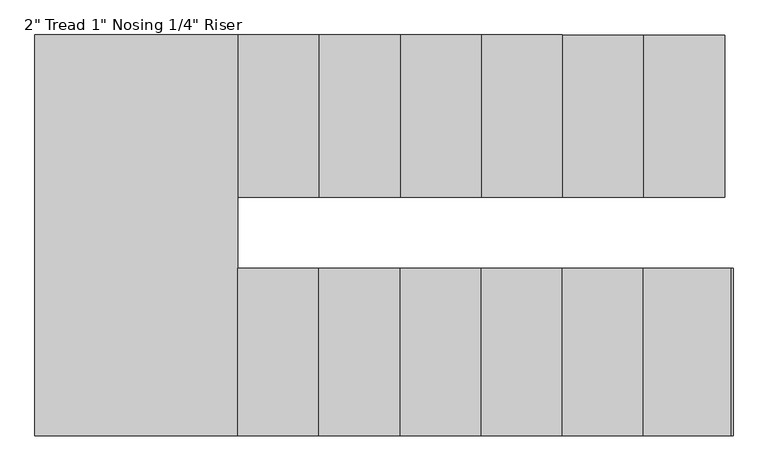
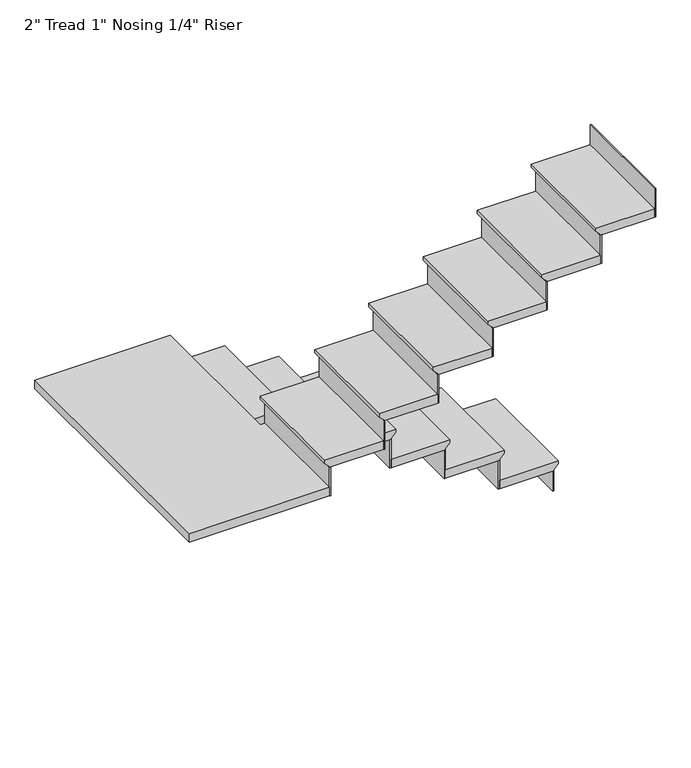
"""IFC4 building model written with IfcOpenShell, lengths in millimetres: stair flight geometry."""

from ifc_helpers import new_model, si_unit, origin, place, context, project, spatial, faceted_brep, source, transform, mapped, element, save


def stair_flight_6f8696f7(model_context):
    return source(origin(), model_context, "Body", "Brep", [
        faceted_brep([(-2968.8120155, -2170.0065691, 6551.0833333), (-2968.8120155, -2170.0065691, 6570.1333333), (-2968.8120155, -2779.6065691, 6570.1333333), (-2968.8120155, -2779.6065691, 6551.0833333), (-2994.2120155, -2170.0065691, 6525.6833333), (-2994.2120155, -2779.6065691, 6525.6833333), (-3299.0120155, -2170.0065691, 6570.1333333), (-3299.0120155, -2779.6065691, 6570.1333333), (-2994.2120155, -2779.6065691, 6519.3333333), (-3299.0120155, -2779.6065691, 6519.3333333), (-3299.0120155, -2170.0065691, 6519.3333333), (-2994.2120155, -2170.0065691, 6519.3333333)], [[[0, 1, 2, 3]], [[4, 0, 3, 5]], [[2, 1, 6, 7]], [[8, 9, 10, 11]], [[2, 7, 9, 8, 5, 3]], [[8, 11, 4, 5]], [[6, 1, 0, 4, 11, 10]], [[7, 6, 10, 9]]]),
        faceted_brep([(-2994.2120155, -2170.0065691, 6519.3333333), (-2994.2120155, -2170.0065691, 6400.8), (-3000.5620155, -2170.0065691, 6400.8), (-3000.5620155, -2170.0065691, 6519.3333333), (-2994.2120155, -2779.6065691, 6519.3333333), (-3000.5620155, -2779.6065691, 6519.3333333), (-3000.5620155, -2779.6065691, 6400.8), (-2994.2120155, -2779.6065691, 6400.8)], [[[0, 1, 2, 3]], [[4, 5, 6, 7]], [[1, 0, 4, 7]], [[2, 1, 7, 6]], [[3, 2, 6, 5]], [[0, 3, 5, 4]]]),
        faceted_brep([(-3299.0120155, -2170.0065691, 6688.6666667), (-3299.0120155, -2170.0065691, 6519.3333333), (-3305.3620155, -2170.0065691, 6519.3333333), (-3305.3620155, -2170.0065691, 6688.6666667), (-3299.0120155, -2779.6065691, 6688.6666667), (-3305.3620155, -2779.6065691, 6688.6666667), (-3305.3620155, -2779.6065691, 6519.3333333), (-3299.0120155, -2779.6065691, 6519.3333333)], [[[0, 1, 2, 3]], [[4, 5, 6, 7]], [[1, 0, 4, 7]], [[2, 1, 7, 6]], [[3, 2, 6, 5]], [[0, 3, 5, 4]]]),
        faceted_brep([(-3273.6120155, -2779.6065691, 6739.4666667), (-3273.6120155, -2170.0065691, 6739.4666667), (-3603.8120155, -2170.0065691, 6739.4666667), (-3603.8120155, -2779.6065691, 6739.4666667), (-3299.0120155, -2779.6065691, 6688.6666667), (-3603.8120155, -2779.6065691, 6688.6666667), (-3603.8120155, -2170.0065691, 6688.6666667), (-3299.0120155, -2170.0065691, 6688.6666667), (-3299.0120155, -2779.6065691, 6695.0166667), (-3273.6120155, -2779.6065691, 6720.4166667), (-3299.0120155, -2170.0065691, 6695.0166667), (-3273.6120155, -2170.0065691, 6720.4166667)], [[[0, 1, 2, 3]], [[4, 5, 6, 7]], [[0, 3, 5, 4, 8, 9]], [[4, 7, 10, 8]], [[2, 1, 11, 10, 7, 6]], [[3, 2, 6, 5]], [[11, 1, 0, 9]], [[10, 11, 9, 8]]]),
        faceted_brep([(-3603.8120155, -2170.0065691, 6858.0), (-3603.8120155, -2170.0065691, 6688.6666667), (-3610.1620155, -2170.0065691, 6688.6666667), (-3610.1620155, -2170.0065691, 6858.0), (-3603.8120155, -2779.6065691, 6858.0), (-3610.1620155, -2779.6065691, 6858.0), (-3610.1620155, -2779.6065691, 6688.6666667), (-3603.8120155, -2779.6065691, 6688.6666667)], [[[0, 1, 2, 3]], [[4, 5, 6, 7]], [[1, 0, 4, 7]], [[2, 1, 7, 6]], [[3, 2, 6, 5]], [[0, 3, 5, 4]]]),
        faceted_brep([(-3578.4120155, -2779.6065691, 6908.8), (-3578.4120155, -2170.0065691, 6908.8), (-3908.6120155, -2170.0065691, 6908.8), (-3908.6120155, -2779.6065691, 6908.8), (-3603.8120155, -2779.6065691, 6858.0), (-3908.6120155, -2779.6065691, 6858.0), (-3908.6120155, -2170.0065691, 6858.0), (-3603.8120155, -2170.0065691, 6858.0), (-3603.8120155, -2779.6065691, 6864.35), (-3578.4120155, -2779.6065691, 6889.75), (-3603.8120155, -2170.0065691, 6864.35), (-3578.4120155, -2170.0065691, 6889.75)], [[[0, 1, 2, 3]], [[4, 5, 6, 7]], [[0, 3, 5, 4, 8, 9]], [[4, 7, 10, 8]], [[2, 1, 11, 10, 7, 6]], [[3, 2, 6, 5]], [[11, 1, 0, 9]], [[10, 11, 9, 8]]]),
        faceted_brep([(-3908.6120155, -2170.0065691, 7027.3333333), (-3908.6120155, -2170.0065691, 6858.0), (-3914.9620155, -2170.0065691, 6858.0), (-3914.9620155, -2170.0065691, 7027.3333333), (-3908.6120155, -2779.6065691, 7027.3333333), (-3914.9620155, -2779.6065691, 7027.3333333), (-3914.9620155, -2779.6065691, 6858.0), (-3908.6120155, -2779.6065691, 6858.0)], [[[0, 1, 2, 3]], [[4, 5, 6, 7]], [[1, 0, 4, 7]], [[2, 1, 7, 6]], [[3, 2, 6, 5]], [[0, 3, 5, 4]]]),
        faceted_brep([(-3883.2120155, -2779.6065691, 7078.1333333), (-3883.2120155, -2170.0065691, 7078.1333333), (-4213.4120155, -2170.0065691, 7078.1333333), (-4213.4120155, -2779.6065691, 7078.1333333), (-3908.6120155, -2779.6065691, 7027.3333333), (-4213.4120155, -2779.6065691, 7027.3333333), (-4213.4120155, -2170.0065691, 7027.3333333), (-3908.6120155, -2170.0065691, 7027.3333333), (-3908.6120155, -2779.6065691, 7033.6833333), (-3883.2120155, -2779.6065691, 7059.0833333), (-3908.6120155, -2170.0065691, 7033.6833333), (-3883.2120155, -2170.0065691, 7059.0833333)], [[[0, 1, 2, 3]], [[4, 5, 6, 7]], [[0, 3, 5, 4, 8, 9]], [[4, 7, 10, 8]], [[2, 1, 11, 10, 7, 6]], [[3, 2, 6, 5]], [[11, 1, 0, 9]], [[10, 11, 9, 8]]]),
        faceted_brep([(-4213.4120155, -2170.0065691, 7196.6666667), (-4213.4120155, -2170.0065691, 7027.3333333), (-4219.7620155, -2170.0065691, 7027.3333333), (-4219.7620155, -2170.0065691, 7196.6666667), (-4213.4120155, -2779.6065691, 7196.6666667), (-4219.7620155, -2779.6065691, 7196.6666667), (-4219.7620155, -2779.6065691, 7027.3333333), (-4213.4120155, -2779.6065691, 7027.3333333)], [[[0, 1, 2, 3]], [[4, 5, 6, 7]], [[1, 0, 4, 7]], [[2, 1, 7, 6]], [[3, 2, 6, 5]], [[0, 3, 5, 4]]]),
        faceted_brep([(-4188.0120155, -2779.6065691, 7247.4666667), (-4188.0120155, -2170.0065691, 7247.4666667), (-4518.2120155, -2170.0065691, 7247.4666667), (-4518.2120155, -2779.6065691, 7247.4666667), (-4213.4120155, -2779.6065691, 7196.6666667), (-4518.2120155, -2779.6065691, 7196.6666667), (-4518.2120155, -2170.0065691, 7196.6666667), (-4213.4120155, -2170.0065691, 7196.6666667), (-4213.4120155, -2779.6065691, 7203.0166667), (-4188.0120155, -2779.6065691, 7228.4166667), (-4213.4120155, -2170.0065691, 7203.0166667), (-4188.0120155, -2170.0065691, 7228.4166667)], [[[0, 1, 2, 3]], [[4, 5, 6, 7]], [[0, 3, 5, 4, 8, 9]], [[4, 7, 10, 8]], [[2, 1, 11, 10, 7, 6]], [[3, 2, 6, 5]], [[11, 1, 0, 9]], [[10, 11, 9, 8]]]),
        faceted_brep([(-4518.2120155, -2170.0065691, 7366.0), (-4518.2120155, -2170.0065691, 7196.6666667), (-4524.5620155, -2170.0065691, 7196.6666667), (-4524.5620155, -2170.0065691, 7366.0), (-4518.2120155, -2779.6065691, 7366.0), (-4524.5620155, -2779.6065691, 7366.0), (-4524.5620155, -2779.6065691, 7196.6666667), (-4518.2120155, -2779.6065691, 7196.6666667)], [[[0, 1, 2, 3]], [[4, 5, 6, 7]], [[1, 0, 4, 7]], [[2, 1, 7, 6]], [[3, 2, 6, 5]], [[0, 3, 5, 4]]]),
        faceted_brep([(-4492.8120155, -2779.6065691, 7416.8), (-4492.8120155, -2170.0065691, 7416.8), (-4823.0120155, -2170.0065691, 7416.8), (-4823.0120155, -2779.6065691, 7416.8), (-4518.2120155, -2779.6065691, 7366.0), (-4823.0120155, -2779.6065691, 7366.0), (-4823.0120155, -2170.0065691, 7366.0), (-4518.2120155, -2170.0065691, 7366.0), (-4518.2120155, -2779.6065691, 7372.35), (-4492.8120155, -2779.6065691, 7397.75), (-4518.2120155, -2170.0065691, 7372.35), (-4492.8120155, -2170.0065691, 7397.75)], [[[0, 1, 2, 3]], [[4, 5, 6, 7]], [[0, 3, 5, 4, 8, 9]], [[4, 7, 10, 8]], [[2, 1, 11, 10, 7, 6]], [[3, 2, 6, 5]], [[11, 1, 0, 9]], [[10, 11, 9, 8]]]),
        faceted_brep([(-4823.0120155, -2170.0065691, 7535.3333333), (-4823.0120155, -2170.0065691, 7366.0), (-4829.3620155, -2170.0065691, 7366.0), (-4829.3620155, -2170.0065691, 7535.3333333), (-4823.0120155, -2779.6065691, 7535.3333333), (-4829.3620155, -2779.6065691, 7535.3333333), (-4829.3620155, -2779.6065691, 7366.0), (-4823.0120155, -2779.6065691, 7366.0)], [[[0, 1, 2, 3]], [[4, 5, 6, 7]], [[1, 0, 4, 7]], [[2, 1, 7, 6]], [[3, 2, 6, 5]], [[0, 3, 5, 4]]]),
        faceted_brep([(-4772.2120155, -3046.3065691, 7586.1333333), (-4797.6120155, -3046.3065691, 7586.1333333), (-4797.6120155, -2170.0065691, 7586.1333333), (-5559.6120155, -2170.0065691, 7586.1333333), (-5559.6120155, -3674.9565691, 7586.1333333), (-4772.2120155, -3674.9565691, 7586.1333333), (-4797.6120155, -3046.3065691, 7535.3333333), (-4772.2120155, -3046.3065691, 7535.3333333), (-4772.2120155, -3674.9565691, 7535.3333333), (-5559.6120155, -3674.9565691, 7535.3333333), (-5559.6120155, -2170.0065691, 7535.3333333), (-4823.0120155, -2170.0065691, 7535.3333333), (-4823.0120155, -2779.6065691, 7535.3333333), (-4797.6120155, -2779.6065691, 7535.3333333), (-4797.6120155, -2779.6065691, 7567.0833333), (-4797.6120155, -2170.0065691, 7567.0833333), (-4823.0120155, -2779.6065691, 7541.6833333), (-4823.0120155, -2170.0065691, 7541.6833333)], [[[0, 1, 2, 3, 4, 5]], [[6, 7, 8, 9, 10, 11, 12, 13]], [[1, 0, 7, 6]], [[2, 1, 6, 13, 14, 15]], [[13, 12, 16, 14]], [[12, 11, 17, 16]], [[3, 2, 15, 17, 11, 10]], [[4, 3, 10, 9]], [[5, 4, 9, 8]], [[0, 5, 8, 7]], [[17, 15, 14, 16]]]),
        faceted_brep([(-4772.2120155, -3674.9565691, 7704.6666667), (-4772.2120155, -3674.9565691, 7535.3333333), (-4765.8620155, -3674.9565691, 7535.3333333), (-4765.8620155, -3674.9565691, 7704.6666667), (-4772.2120155, -3046.3065691, 7704.6666667), (-4765.8620155, -3046.3065691, 7704.6666667), (-4765.8620155, -3046.3065691, 7535.3333333), (-4772.2120155, -3046.3065691, 7535.3333333)], [[[0, 1, 2, 3]], [[4, 5, 6, 7]], [[1, 0, 4, 7]], [[2, 1, 7, 6]], [[3, 2, 6, 5]], [[0, 3, 5, 4]]]),
        faceted_brep([(-4797.6120155, -3046.3065691, 7755.4666667), (-4797.6120155, -3674.9565691, 7755.4666667), (-4467.4120155, -3674.9565691, 7755.4666667), (-4467.4120155, -3046.3065691, 7755.4666667), (-4772.2120155, -3046.3065691, 7704.6666667), (-4467.4120155, -3046.3065691, 7704.6666667), (-4467.4120155, -3674.9565691, 7704.6666667), (-4772.2120155, -3674.9565691, 7704.6666667), (-4772.2120155, -3046.3065691, 7711.0166667), (-4797.6120155, -3046.3065691, 7736.4166667), (-4772.2120155, -3674.9565691, 7711.0166667), (-4797.6120155, -3674.9565691, 7736.4166667)], [[[0, 1, 2, 3]], [[4, 5, 6, 7]], [[0, 3, 5, 4, 8, 9]], [[4, 7, 10, 8]], [[2, 1, 11, 10, 7, 6]], [[3, 2, 6, 5]], [[11, 1, 0, 9]], [[10, 11, 9, 8]]]),
        faceted_brep([(-4467.4120155, -3674.9565691, 7874.0), (-4467.4120155, -3674.9565691, 7704.6666667), (-4461.0620155, -3674.9565691, 7704.6666667), (-4461.0620155, -3674.9565691, 7874.0), (-4467.4120155, -3046.3065691, 7874.0), (-4461.0620155, -3046.3065691, 7874.0), (-4461.0620155, -3046.3065691, 7704.6666667), (-4467.4120155, -3046.3065691, 7704.6666667)], [[[0, 1, 2, 3]], [[4, 5, 6, 7]], [[1, 0, 4, 7]], [[2, 1, 7, 6]], [[3, 2, 6, 5]], [[0, 3, 5, 4]]]),
        faceted_brep([(-4492.8120155, -3046.3065691, 7924.8), (-4492.8120155, -3674.9565691, 7924.8), (-4162.6120155, -3674.9565691, 7924.8), (-4162.6120155, -3046.3065691, 7924.8), (-4467.4120155, -3046.3065691, 7874.0), (-4162.6120155, -3046.3065691, 7874.0), (-4162.6120155, -3674.9565691, 7874.0), (-4467.4120155, -3674.9565691, 7874.0), (-4467.4120155, -3046.3065691, 7880.35), (-4492.8120155, -3046.3065691, 7905.75), (-4467.4120155, -3674.9565691, 7880.35), (-4492.8120155, -3674.9565691, 7905.75)], [[[0, 1, 2, 3]], [[4, 5, 6, 7]], [[0, 3, 5, 4, 8, 9]], [[4, 7, 10, 8]], [[2, 1, 11, 10, 7, 6]], [[3, 2, 6, 5]], [[11, 1, 0, 9]], [[10, 11, 9, 8]]]),
        faceted_brep([(-4162.6120155, -3674.9565691, 8043.3333333), (-4162.6120155, -3674.9565691, 7874.0), (-4156.2620155, -3674.9565691, 7874.0), (-4156.2620155, -3674.9565691, 8043.3333333), (-4162.6120155, -3046.3065691, 8043.3333333), (-4156.2620155, -3046.3065691, 8043.3333333), (-4156.2620155, -3046.3065691, 7874.0), (-4162.6120155, -3046.3065691, 7874.0)], [[[0, 1, 2, 3]], [[4, 5, 6, 7]], [[1, 0, 4, 7]], [[2, 1, 7, 6]], [[3, 2, 6, 5]], [[0, 3, 5, 4]]]),
        faceted_brep([(-4188.0120155, -3046.3065691, 8094.1333333), (-4188.0120155, -3674.9565691, 8094.1333333), (-3857.8120155, -3674.9565691, 8094.1333333), (-3857.8120155, -3046.3065691, 8094.1333333), (-4162.6120155, -3046.3065691, 8043.3333333), (-3857.8120155, -3046.3065691, 8043.3333333), (-3857.8120155, -3674.9565691, 8043.3333333), (-4162.6120155, -3674.9565691, 8043.3333333), (-4162.6120155, -3046.3065691, 8049.6833333), (-4188.0120155, -3046.3065691, 8075.0833333), (-4162.6120155, -3674.9565691, 8049.6833333), (-4188.0120155, -3674.9565691, 8075.0833333)], [[[0, 1, 2, 3]], [[4, 5, 6, 7]], [[0, 3, 5, 4, 8, 9]], [[4, 7, 10, 8]], [[2, 1, 11, 10, 7, 6]], [[3, 2, 6, 5]], [[11, 1, 0, 9]], [[10, 11, 9, 8]]]),
        faceted_brep([(-3857.8120155, -3674.9565691, 8212.6666667), (-3857.8120155, -3674.9565691, 8043.3333333), (-3851.4620155, -3674.9565691, 8043.3333333), (-3851.4620155, -3674.9565691, 8212.6666667), (-3857.8120155, -3046.3065691, 8212.6666667), (-3851.4620155, -3046.3065691, 8212.6666667), (-3851.4620155, -3046.3065691, 8043.3333333), (-3857.8120155, -3046.3065691, 8043.3333333)], [[[0, 1, 2, 3]], [[4, 5, 6, 7]], [[1, 0, 4, 7]], [[2, 1, 7, 6]], [[3, 2, 6, 5]], [[0, 3, 5, 4]]]),
        faceted_brep([(-3883.2120155, -3046.3065691, 8263.4666667), (-3883.2120155, -3674.9565691, 8263.4666667), (-3553.0120155, -3674.9565691, 8263.4666667), (-3553.0120155, -3046.3065691, 8263.4666667), (-3857.8120155, -3046.3065691, 8212.6666667), (-3553.0120155, -3046.3065691, 8212.6666667), (-3553.0120155, -3674.9565691, 8212.6666667), (-3857.8120155, -3674.9565691, 8212.6666667), (-3857.8120155, -3046.3065691, 8219.0166667), (-3883.2120155, -3046.3065691, 8244.4166667), (-3857.8120155, -3674.9565691, 8219.0166667), (-3883.2120155, -3674.9565691, 8244.4166667)], [[[0, 1, 2, 3]], [[4, 5, 6, 7]], [[0, 3, 5, 4, 8, 9]], [[4, 7, 10, 8]], [[2, 1, 11, 10, 7, 6]], [[3, 2, 6, 5]], [[11, 1, 0, 9]], [[10, 11, 9, 8]]]),
        faceted_brep([(-3553.0120155, -3674.9565691, 8382.0), (-3553.0120155, -3674.9565691, 8212.6666667), (-3546.6620155, -3674.9565691, 8212.6666667), (-3546.6620155, -3674.9565691, 8382.0), (-3553.0120155, -3046.3065691, 8382.0), (-3546.6620155, -3046.3065691, 8382.0), (-3546.6620155, -3046.3065691, 8212.6666667), (-3553.0120155, -3046.3065691, 8212.6666667)], [[[0, 1, 2, 3]], [[4, 5, 6, 7]], [[1, 0, 4, 7]], [[2, 1, 7, 6]], [[3, 2, 6, 5]], [[0, 3, 5, 4]]]),
        faceted_brep([(-3578.4120155, -3046.3065691, 8432.8), (-3578.4120155, -3674.9565691, 8432.8), (-3248.2120155, -3674.9565691, 8432.8), (-3248.2120155, -3046.3065691, 8432.8), (-3553.0120155, -3046.3065691, 8382.0), (-3248.2120155, -3046.3065691, 8382.0), (-3248.2120155, -3674.9565691, 8382.0), (-3553.0120155, -3674.9565691, 8382.0), (-3553.0120155, -3046.3065691, 8388.35), (-3578.4120155, -3046.3065691, 8413.75), (-3553.0120155, -3674.9565691, 8388.35), (-3578.4120155, -3674.9565691, 8413.75)], [[[0, 1, 2, 3]], [[4, 5, 6, 7]], [[0, 3, 5, 4, 8, 9]], [[4, 7, 10, 8]], [[2, 1, 11, 10, 7, 6]], [[3, 2, 6, 5]], [[11, 1, 0, 9]], [[10, 11, 9, 8]]]),
        faceted_brep([(-3248.2120155, -3674.9565691, 8551.3333333), (-3248.2120155, -3674.9565691, 8382.0), (-3241.8620155, -3674.9565691, 8382.0), (-3241.8620155, -3674.9565691, 8551.3333333), (-3248.2120155, -3046.3065691, 8551.3333333), (-3241.8620155, -3046.3065691, 8551.3333333), (-3241.8620155, -3046.3065691, 8382.0), (-3248.2120155, -3046.3065691, 8382.0)], [[[0, 1, 2, 3]], [[4, 5, 6, 7]], [[1, 0, 4, 7]], [[2, 1, 7, 6]], [[3, 2, 6, 5]], [[0, 3, 5, 4]]]),
        faceted_brep([(-2943.4120155, -3674.9565691, 8720.6666667), (-2943.4120155, -3674.9565691, 8551.3333333), (-2937.0620155, -3674.9565691, 8551.3333333), (-2937.0620155, -3674.9565691, 8720.6666667), (-2943.4120155, -3046.3065691, 8720.6666667), (-2937.0620155, -3046.3065691, 8720.6666667), (-2937.0620155, -3046.3065691, 8551.3333333), (-2943.4120155, -3046.3065691, 8551.3333333)], [[[0, 1, 2, 3]], [[4, 5, 6, 7]], [[1, 0, 4, 7]], [[2, 1, 7, 6]], [[3, 2, 6, 5]], [[0, 3, 5, 4]]]),
        faceted_brep([(-3273.6120155, -3046.3065691, 8602.1333333), (-3273.6120155, -3674.9565691, 8602.1333333), (-2943.4120155, -3674.9565691, 8602.1333333), (-2943.4120155, -3046.3065691, 8602.1333333), (-3248.2120155, -3046.3065691, 8551.3333333), (-2943.4120155, -3046.3065691, 8551.3333333), (-2943.4120155, -3674.9565691, 8551.3333333), (-3248.2120155, -3674.9565691, 8551.3333333), (-3248.2120155, -3046.3065691, 8557.6833333), (-3273.6120155, -3046.3065691, 8583.0833333), (-3248.2120155, -3674.9565691, 8557.6833333), (-3273.6120155, -3674.9565691, 8583.0833333)], [[[0, 1, 2, 3]], [[4, 5, 6, 7]], [[0, 3, 5, 4, 8, 9]], [[4, 7, 10, 8]], [[2, 1, 11, 10, 7, 6]], [[3, 2, 6, 5]], [[11, 1, 0, 9]], [[10, 11, 9, 8]]]),
    ])


if __name__ == "__main__":
    model = new_model("IFC4")
    model_context = context("Model", 3, world=origin())
    ifc_project = project(units=[si_unit("LENGTHUNIT", "METRE", prefix="MILLI")], contexts=[model_context])
    site = spatial("IfcSite", under=ifc_project)
    building = spatial("IfcBuilding", under=site)
    placement = place(None, origin())
    stair_flight_shape = stair_flight_6f8696f7(model_context)
    element("IfcStairFlight", 1, ObjectType="2\" Tread 1\" Nosing 1/4\" Riser", at=placement, inside=building, context=model_context, shape_type="MappedRepresentation", body=[
        mapped(stair_flight_shape, transform((0.0, 0.0, 0.0), x_axis=(1.0, 0.0, 0.0), y_axis=(0.0, 1.0, 0.0), z_axis=(0.0, 0.0, 1.0))),
    ])
    save(model, "model.ifc")
